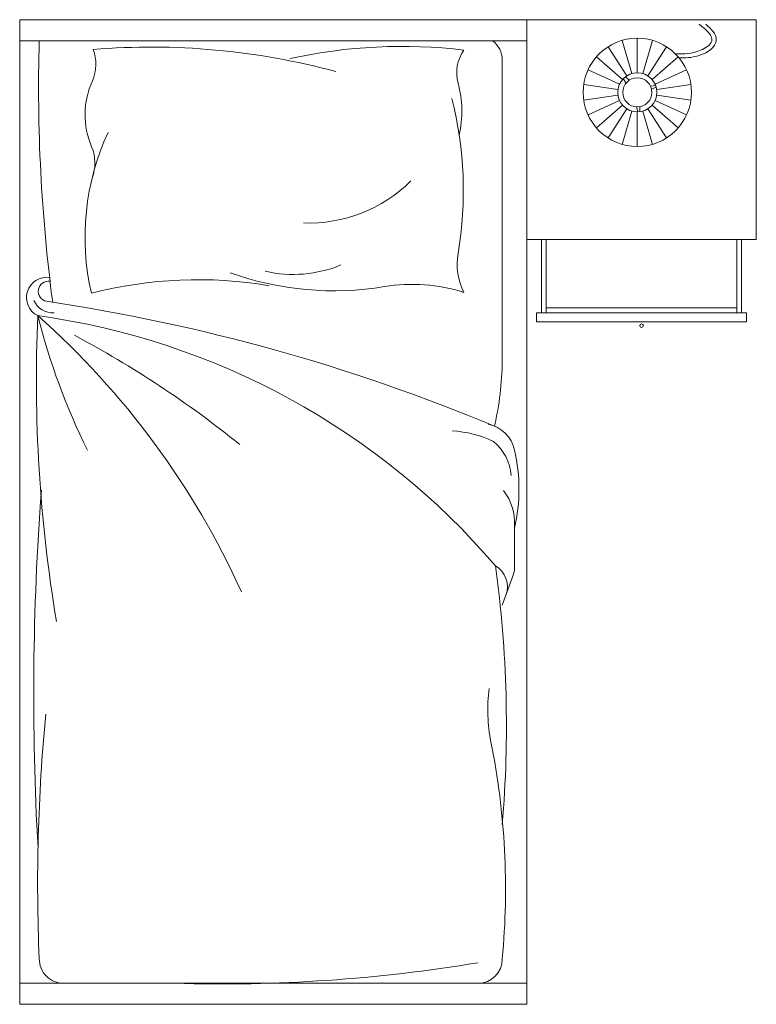
# Model space of a CAD drawing. Units: inches. Extents: x 1994 to 3075, y 3517 to 3950.
# Tile 13 of 58: x 1994.32591 to 1994.38458, y 3553.47149 to 3553.5499. Entities that reach past the tile are written whole.
import ezdxf

# ---------------------------------------------------------------- set-up
doc = ezdxf.new("R2010")
doc.units = ezdxf.units.IN
doc.layers.add('A-FURN-REFR', color=8, linetype='Continuous', lineweight=13)

msp = doc.modelspace()

# ---------------------------------------------------------------- linework, layer by layer
at = {"layer": 'A-FURN-REFR'}
for p, q in [((1994.366294088309, 3553.549896824299), (1994.325909174557, 3553.549896824299)), ((1994.325909174557, 3553.549896824299), (1994.325909174541, 3553.471489836036)), ((1994.366294088309, 3553.549896824299), (1994.366294088293, 3553.471489836036)), ((1994.384582566965, 3553.549896824306), (1994.366294088309, 3553.549896824306)), ((1994.384582566965, 3553.532386578792), (1994.384582566965, 3553.549896824306)), ((1994.325909174557, 3553.548223623056), (1994.366294088309, 3553.548223623042)), ((1994.373887758048, 3553.54825191407), (1994.374663344528, 3553.54561050909)), ((1994.375103829025, 3553.54842675868), (1994.375103829025, 3553.545673841199)), ((1994.375103829025, 3553.54842675868), (1994.375103829025, 3553.545673841199)), ((1994.376319900003, 3553.54825191407), (1994.375544313522, 3553.54561050909)), ((1994.374258545466, 3553.545425643552), (1994.372770205909, 3553.547741545109)), ((1994.377437452142, 3553.547741545109), (1994.375949112585, 3553.545425643552)), ((1994.364348505468, 3553.522716254859), (1994.364348505473, 3553.546667156793)), ((1994.373922226251, 3553.545134221293), (1994.371841710036, 3553.546936998856)), ((1994.378365948015, 3553.546936998856), (1994.3762854318, 3553.545134221293)), ((1994.373681633464, 3553.54475985161), (1994.371177491643, 3553.545903454862)), ((1994.379030166408, 3553.545903454862), (1994.376526024586, 3553.54475985161)), ((1994.374209203992, 3553.544846356139), (1994.373984953241, 3553.545202419334)), ((1994.374491805488, 3553.545093960428), (1994.374134179373, 3553.545336840846)), ((1994.373556258505, 3553.54433286371), (1994.370831361754, 3553.544724644716)), ((1994.376156047634, 3553.544595006205), (1994.376566276772, 3553.544663285672)), ((1994.376235176752, 3553.544359558391), (1994.376611144457, 3553.544525668704)), ((1994.379376296296, 3553.544724644716), (1994.376651399546, 3553.54433286371)), ((1994.373556258505, 3553.543887849611), (1994.370831361754, 3553.543496068605)), ((1994.379376296296, 3553.543496068605), (1994.376651399546, 3553.543887849611)), ((1994.373681633464, 3553.54346086171), (1994.371177491643, 3553.54231725846)), ((1994.373922226251, 3553.543086492028), (1994.371841710036, 3553.541283714466)), ((1994.374258545466, 3553.542795069769), (1994.372770205909, 3553.540479168212)), ((1994.375046107135, 3553.542953327117), (1994.375148102379, 3553.542547499094)), ((1994.375314391896, 3553.54297118483), (1994.375311543915, 3553.542560731407)), ((1994.377437452142, 3553.540479168212), (1994.375949112585, 3553.542795069769)), ((1994.378365948015, 3553.541283714466), (1994.3762854318, 3553.543086492028)), ((1994.379030166408, 3553.54231725846), (1994.376526024586, 3553.54346086171)), ((1994.374663344528, 3553.542610204231), (1994.373887758048, 3553.539968799251)), ((1994.375103829025, 3553.542546872122), (1994.375103829025, 3553.53979395464)), ((1994.375103829025, 3553.542546872122), (1994.375103829025, 3553.53979395464)), ((1994.375544313522, 3553.542610204231), (1994.376319900003, 3553.539968799251)), ((1994.366294088313, 3553.532386578788), (1994.384582566965, 3553.532386578792)), ((1994.367461438014, 3553.532386578788), (1994.367461438015, 3553.526549830281)), ((1994.367850554581, 3553.532386578788), (1994.367850554582, 3553.526549830282)), ((1994.383026100697, 3553.532386578791), (1994.383026100698, 3553.526549830286)), ((1994.383415217264, 3553.532386578791), (1994.383415217265, 3553.526549830286)), ((1994.367072321448, 3553.526549830281), (1994.383804333832, 3553.526549830286)), ((1994.367072321449, 3553.525849420462), (1994.367072321448, 3553.526549830281)), ((1994.383026100698, 3553.526938946852), (1994.367850554582, 3553.526938946849)), ((1994.383804333832, 3553.526549830286), (1994.383804333832, 3553.525849420465)), ((1994.383804333832, 3553.525849420465), (1994.367072321449, 3553.525849420462)), ((1994.365321296883, 3553.506268617844), (1994.365321296884, 3553.510086444833)), ((1994.365201091204, 3553.505595349098), (1994.364348505465, 3553.503283804798)), ((1994.325909174541, 3553.473163037264), (1994.366294088294, 3553.473163037255)), ((1994.325909174557, 3553.471489836036), (1994.366294088293, 3553.471489836036))]:
    msp.add_line(p, q, dxfattribs=at)
for radius in [0.0043164020201009, 0.0015634845390022, 0.0011584684638608]:
    msp.add_circle((1994.375103829025, 3553.544110356661), radius, dxfattribs=at)
for centre, radius, start, end in [((1994.457982307409, 3553.544510292255), 0.1305694799013457, 178.3703169121375, 187.5322278354393), ((1994.362402922638, 3553.546667156793), 0.0019455828353276, 359.9999999880876, 53.13010234330246), ((1994.328778192757, 3553.54634209869), 0.0032028341489732, 335.7877323280015, 21.71237864400314), ((1994.336366123564, 3553.491209131769), 0.0565064023996118, 74.89247536308716, 94.681970907379), ((1994.356345820335, 3553.506299895526), 0.0414680575843914, 83.14136388124066, 102.4247502365447), ((1994.363823990246, 3553.54566130914), 0.0031075126812102, 144.3787648229011, 195.1987658355305), ((1994.337697232182, 3553.542331427842), 0.0065764677133891, 155.7877323280015, 202.8808293159797), ((1994.352529572374, 3553.542592944963), 0.0085962787467616, 347.311957921453, 15.19876583553051), ((1994.331389969925, 3553.536279099003), 0.0298558147000044, 350.3711224665587, 14.25995084780135), ((1994.350964373986, 3553.532568198205), 0.0198519972069101, 155.1179531461462, 192.9861889591517), ((1994.328560863893, 3553.538475676689), 0.0033401870886801, 339.0160855821216, 22.88082931597971), ((1994.348958297249, 3553.545159879192), 0.0114567055564695, 267.8294752673963, 315.0098308273483), ((1994.365750874456, 3553.530449571898), 0.004996088352876, 170.3711224665586, 206.9649370961853), ((1994.347694574241, 3553.539599281242), 0.009989213432703, 257.148031947205, 292.3825063085086), ((1994.328058800165, 3553.527774762038), 0.0016105685091622, 81.6091039781453, 243.938180591863), ((1994.350952768637, 3553.552948825775), 0.0246390736856652, 250.3559327023518, 279.3925899659531), ((1994.328206047761, 3553.528265221731), 0.0008128892221172, 81.29146871137522, 258.1255955891823), ((1994.340112618823, 3553.495497603466), 0.0336972432594088, 80.32657587842615, 104.5973118255227), ((1994.357187471541, 3553.515257787318), 0.0135641447689492, 72.35976010254194, 99.39258996595309), ((1994.328526803205, 3553.528161241527), 0.0016095821071006, 202.6051908922757, 274.4988817166678), ((1994.306253237658, 3553.380291995377), 0.1487813656996577, 67.27623853958569, 81.58010286503209), ((1994.443867994845, 3553.521228643783), 0.1166283141987217, 177.4940716817132, 189.5094068679036), ((1994.283880830742, 3553.477274337105), 0.065543355857517, 24.38326925012849, 48.45324971012612), ((1994.319325911715, 3553.468323236192), 0.0585572615340703, 40.58068443299209, 82.12279458076166), ((1994.379790342996, 3553.539586758712), 0.0540893550839264, 194.1893851607317, 206.3095844034524), ((1994.37543832764, 3553.525531922741), 0.00014591871265, 1.19123935e-08, 180.0000000119124), ((1994.37543832764, 3553.525531922741), 0.00014591871265, 180.0000000119124, 1.19123935e-08), ((1994.291899782341, 3553.452348197666), 0.0819509525067612, 51.03759283326017, 62.08562985249065), ((1994.33963120898, 3553.523047893384), 0.0247195212287987, 347.0890423172248, 359.2312934508153), ((1994.362676268209, 3553.515011147364), 0.0027238159694586, 12.88269036848606, 78.38686031445394), ((1994.359786020217, 3553.508040224145), 0.0091331594194461, 65.03385580996276, 86.4640048798947), ((1994.361139029012, 3553.513274218948), 0.0039416012902181, 4.684898432501862, 50.59840531545589), ((1994.351851412719, 3553.512535366099), 0.013828183994568, 346.9286456497866, 12.88269036848606), ((1994.543836828317, 3553.496154656567), 0.2168115609509192, 175.697202442643, 183.2229785434103), ((1994.361134108863, 3553.509837803962), 0.0041945638393764, 356.601689895136, 37.73019638534235), ((1994.271499874226, 3553.493646793476), 0.0931787946855045, 355.1752823324409, 7.876466900264919), ((1994.362811772672, 3553.504739650832), 0.0019455828353278, 339.7541012352643, 59.48721857724742), ((1994.363375714047, 3553.506268617845), 0.0019455828353276, 339.7541012352643, 359.9999999880876), ((1994.363375714047, 3553.506268617845), 0.0019455828353276, 339.7541012352643, 359.9999999880876), ((1994.376167648434, 3553.494933181291), 0.0129749866847535, 172.4746658505032, 191.3425348756069), ((1994.46862867607, 3553.481090515266), 0.1412897221787423, 174.5126540947314, 182.4265021931356), ((1994.305069481107, 3553.480671468557), 0.0595394659951302, 354.6389628949611, 11.34253487560691), ((1994.329411223645, 3553.475108620109), 0.0019455828353276, 179.9999999880876, 269.9999999880876), ((1994.341953700146, 3553.597248944618), 0.1241401229318277, 268.3066004926072, 279.4831521227457), ((1994.362402922623, 3553.47510862011), 0.0019455828353276, 269.9999999880876, 359.9999999880876)]:
    msp.add_arc(centre, radius, start, end, dxfattribs=at)
for points, knots in [([(1994.378140828596, 3553.547177596464), (1994.378794077944, 3553.547165363887), (1994.379816549943, 3553.547158526936), (1994.381543704804, 3553.548283053891), (1994.38060001375, 3553.54907497106), (1994.380034564405, 3553.549542607669)], [0, 0, 0, 0, 0.0020194675198324, 0.0031659294015444, 0.0048546887782932, 0.0048546887782932, 0.0048546887782932, 0.0048546887782932]), ([(1994.378441471096, 3553.546847411978), (1994.378913720666, 3553.546843562644), (1994.379414958061, 3553.546863829855), (1994.380481607302, 3553.547196998869), (1994.381153690143, 3553.547448726718), (1994.381515464158, 3553.548603285282), (1994.381115494867, 3553.54902355939), (1994.380669875472, 3553.549431438474), (1994.380606283854, 3553.549487295226), (1994.380541769018, 3553.549542607669)], [0.0077183477163671, 0.0077183477163671, 0.0077183477163671, 0.0077183477163671, 0.0428867239757183, 0.0428867239757183, 0.0785443346356031, 0.0785443346356031, 0.1084777623087474, 0.1084777623087474, 0.1132872864949097, 0.1132872864949097, 0.1132872864949097, 0.1132872864949097])]:
    msp.add_open_spline(points, degree=3, knots=knots, dxfattribs=at)

doc.saveas('drawing.dxf')
